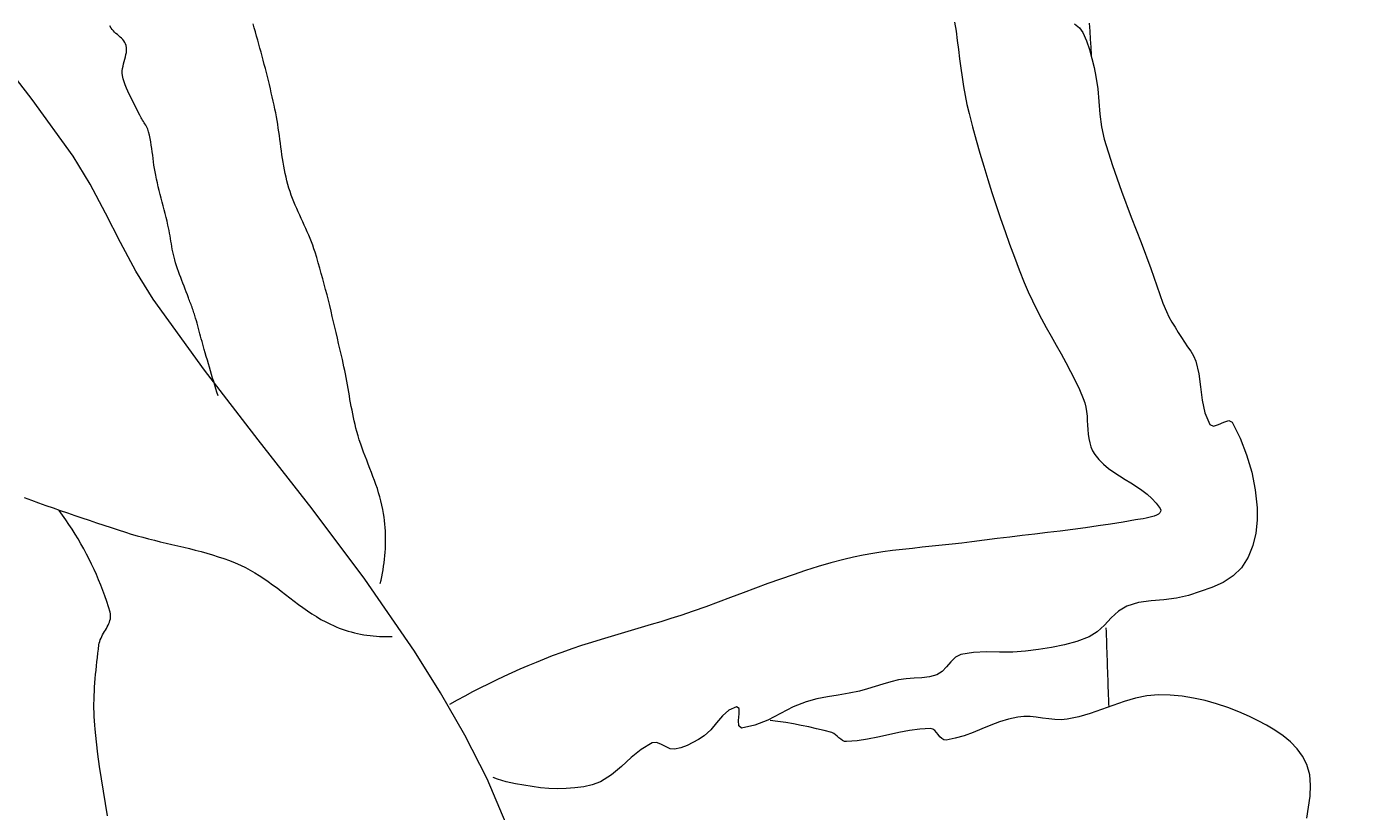
# Model space of a CAD drawing. Units: inches. Extents: x 1441 to 2460, y 1648 to 2683.
# Tile 7 of 35: x 1852 to 1880, y 1901 to 1917. Entities that reach past the tile are written whole.
import ezdxf

# ---------------------------------------------------------------- set-up
doc = ezdxf.new("R2010")
doc.units = ezdxf.units.IN
doc.layers.add('A-ANNO-DIMS', color=2, linetype='Continuous', lineweight=18)
doc.layers.add('A-FURN', color=8, linetype='Continuous', lineweight=15)
doc.styles.get("Standard").update_dxf_attribs({"font": 'arial.ttf'})
doc.dimstyles.get("Standard").update_dxf_attribs({"dimtxt": 0.18, "dimasz": 0.18, "dimexe": 0.18, "dimexo": 0.0625, "dimgap": 0.09, "dimtad": 0, "dimtih": 1, "dimtoh": 1, "dimdec": 4, "dimzin": 0, "dimdsep": 46, "dimtxsty": 'Standard', "dimcen": 0.09, "dimadec": 0, "dimazin": 0, "dimtfac": 1, "dimtdec": 4, "dimtofl": 0, "dimtmove": 0, "dimatfit": 3, "dimfxl": 1, "dimtolj": 1, "dimtzin": 0, "dimarcsym": 0})

# ---------------------------------------------------------------- blocks, each defined once
blk = doc.blocks.new('BED-DOUBLE-PLAN')
for p, q in [((30.489, 90.832), (30.333, 90.717)), ((30.661, 90.921), (30.489, 90.832)), ((30.874, 90.983), (30.661, 90.921)), ((31.094, 91.001), (30.874, 90.983)), ((31.32, 90.99), (31.094, 91.001)), ((31.549, 90.959), (31.32, 90.99)), ((31.78, 90.922), (31.549, 90.959)), ((30.192, 90.579), (30.063, 90.425)), ((30.333, 90.717), (30.192, 90.579)), ((29.947, 90.257), (29.842, 90.082)), ((30.063, 90.425), (29.947, 90.257)), ((29.842, 90.082), (29.747, 89.903)), ((23.852, 89.529), (24.202, 89.666)), ((24.202, 89.666), (24.563, 89.771)), ((24.563, 89.771), (24.931, 89.844)), ((24.931, 89.844), (25.302, 89.885)), ((25.302, 89.885), (25.565, 89.887)), ((25.565, 89.887), (25.831, 89.859)), ((25.831, 89.859), (26.09, 89.797)), ((26.09, 89.797), (26.334, 89.698)), ((26.334, 89.698), (26.554, 89.56)), ((29.66, 89.724), (29.561, 89.501)), ((29.747, 89.903), (29.66, 89.724)), ((23.52, 89.361), (23.852, 89.529)), ((26.554, 89.56), (26.727, 89.384)), ((26.727, 89.384), (26.861, 89.173)), ((29.561, 89.501), (29.471, 89.271)), ((23.486, 89.292), (23.52, 89.361)), ((23.516, 89.189), (23.486, 89.292)), ((23.569, 89.075), (23.516, 89.189)), ((26.861, 89.173), (26.965, 88.94)), ((29.471, 89.271), (29.393, 89.037)), ((23.32, 88.794), (23.566, 88.9)), ((23.566, 88.9), (23.6, 88.971)), ((23.6, 88.971), (23.569, 89.075)), ((26.965, 88.94), (27.052, 88.696)), ((29.393, 89.037), (29.327, 88.8)), ((22.037, 88.5), (22.136, 88.557)), ((22.136, 88.557), (22.241, 88.602)), ((22.241, 88.602), (22.507, 88.665)), ((22.507, 88.665), (22.781, 88.701)), ((22.781, 88.701), (23.055, 88.736)), ((23.055, 88.736), (23.32, 88.794)), ((27.052, 88.696), (27.132, 88.454)), ((29.274, 88.559), (29.236, 88.317)), ((29.327, 88.8), (29.274, 88.559)), ((21.643, 88.24), (21.75, 88.305)), ((21.75, 88.305), (21.847, 88.368)), ((21.847, 88.368), (21.942, 88.434)), ((21.942, 88.434), (22.037, 88.5)), ((27.132, 88.454), (27.192, 88.199)), ((29.236, 88.317), (29.214, 88.073)), ((21.031, 87.917), (21.207, 87.99)), ((21.207, 87.99), (21.32, 88.045)), ((21.32, 88.045), (21.429, 88.107)), ((21.429, 88.107), (21.536, 88.173)), ((21.536, 88.173), (21.643, 88.24)), ((27.192, 88.199), (27.223, 87.936)), ((29.214, 88.073), (29.208, 87.829)), ((20.309, 87.666), (20.489, 87.729)), ((20.489, 87.729), (20.67, 87.789)), ((20.67, 87.789), (20.851, 87.851)), ((20.851, 87.851), (21.031, 87.917)), ((25.019, 87.589), (25.108, 87.69)), ((25.108, 87.69), (25.206, 87.78)), ((25.206, 87.78), (25.316, 87.859)), ((25.316, 87.859), (25.351, 87.873)), ((25.351, 87.873), (25.382, 87.87)), ((25.382, 87.87), (25.41, 87.854)), ((25.41, 87.854), (25.435, 87.824)), ((25.435, 87.824), (25.457, 87.785)), ((25.457, 87.785), (25.476, 87.737)), ((25.476, 87.737), (25.493, 87.683)), ((27.223, 87.936), (27.246, 87.672)), ((29.208, 87.829), (29.229, 87.585)), ((19.236, 87.259), (19.771, 87.466)), ((19.771, 87.466), (20.309, 87.666)), ((24.859, 87.366), (24.936, 87.481)), ((24.936, 87.481), (25.019, 87.589)), ((25.493, 87.683), (25.508, 87.626)), ((25.508, 87.626), (25.521, 87.566)), ((25.521, 87.566), (25.532, 87.506)), ((25.532, 87.506), (25.542, 87.449)), ((25.542, 87.449), (25.551, 87.396)), ((27.246, 87.672), (27.284, 87.412)), ((27.284, 87.412), (27.359, 87.162)), ((29.229, 87.585), (29.278, 87.345)), ((18.7, 87.056), (19.236, 87.259)), ((24.638, 87.01), (24.712, 87.129)), ((24.712, 87.129), (24.785, 87.248)), ((24.785, 87.248), (24.859, 87.366)), ((25.551, 87.396), (25.559, 87.349)), ((25.559, 87.349), (25.604, 87.088)), ((27.359, 87.162), (27.462, 86.991)), ((29.278, 87.345), (29.347, 87.108)), ((17.613, 86.694), (18.16, 86.865)), ((18.16, 86.865), (18.7, 87.056)), ((24.481, 86.782), (24.562, 86.894)), ((24.562, 86.894), (24.638, 87.01)), ((25.604, 87.088), (25.646, 86.826)), ((27.462, 86.991), (27.601, 86.84)), ((29.347, 87.108), (29.428, 86.873)), ((29.428, 86.873), (29.514, 86.638)), ((16.564, 86.559), (16.828, 86.583)), ((16.828, 86.583), (17.093, 86.605)), ((17.093, 86.605), (17.356, 86.638)), ((17.356, 86.638), (17.613, 86.694)), ((24.194, 86.499), (24.299, 86.583)), ((24.299, 86.583), (24.394, 86.678)), ((24.394, 86.678), (24.481, 86.782)), ((25.646, 86.826), (25.684, 86.564)), ((27.601, 86.84), (27.752, 86.698)), ((27.752, 86.698), (27.893, 86.548)), ((27.813, 86.729), (27.896, 86.732)), ((27.896, 86.732), (27.979, 86.735)), ((27.979, 86.735), (28.061, 86.738)), ((28.061, 86.738), (28.144, 86.741)), ((28.144, 86.741), (28.226, 86.744)), ((28.226, 86.744), (28.309, 86.746)), ((28.309, 86.746), (28.391, 86.749)), ((28.391, 86.749), (28.474, 86.752)), ((28.474, 86.752), (28.556, 86.755)), ((28.556, 86.755), (28.639, 86.758)), ((28.639, 86.758), (28.722, 86.761)), ((28.722, 86.761), (28.804, 86.764)), ((28.804, 86.764), (28.887, 86.767)), ((28.887, 86.767), (28.969, 86.77)), ((28.969, 86.77), (29.052, 86.772)), ((29.052, 86.772), (29.134, 86.775)), ((29.134, 86.775), (29.217, 86.778)), ((29.217, 86.778), (29.3, 86.781)), ((29.3, 86.781), (29.382, 86.784)), ((29.382, 86.784), (29.465, 86.787)), ((29.514, 86.638), (29.596, 86.402)), ((15.193, 86.382), (15.36, 86.392)), ((15.36, 86.392), (15.527, 86.401)), ((15.385, 86.249), (15.56, 86.325)), ((15.527, 86.401), (15.694, 86.411)), ((15.56, 86.325), (15.741, 86.387)), ((15.694, 86.411), (15.86, 86.42)), ((15.741, 86.387), (15.927, 86.438)), ((15.927, 86.438), (16.114, 86.481)), ((16.114, 86.481), (16.302, 86.52)), ((16.302, 86.52), (16.564, 86.559)), ((23.026, 86.257), (23.113, 86.287)), ((23.113, 86.287), (23.203, 86.309)), ((23.203, 86.309), (23.295, 86.324)), ((23.295, 86.324), (23.389, 86.334)), ((23.389, 86.334), (23.483, 86.34)), ((23.483, 86.34), (23.578, 86.346)), ((23.578, 86.346), (23.673, 86.352)), ((23.673, 86.352), (23.767, 86.361)), ((23.767, 86.361), (23.858, 86.373)), ((23.858, 86.373), (23.948, 86.391)), ((23.948, 86.391), (24.034, 86.417)), ((24.034, 86.417), (24.116, 86.452)), ((24.116, 86.452), (24.194, 86.499)), ((25.684, 86.564), (25.721, 86.301)), ((25.721, 86.301), (25.756, 86.038)), ((27.893, 86.548), (28, 86.378)), ((28, 86.378), (28.096, 86.124)), ((29.596, 86.402), (29.666, 86.164)), ((15.205, 86.075), (15.287, 86.175)), ((15.287, 86.175), (15.385, 86.249)), ((22.459, 85.991), (22.646, 86.085)), ((22.646, 86.085), (22.835, 86.174)), ((22.835, 86.174), (23.026, 86.257)), ((25.756, 86.038), (25.789, 85.775)), ((28.096, 86.124), (28.167, 85.862)), ((29.666, 86.164), (29.717, 85.922)), ((21.908, 85.69), (22.091, 85.792)), ((22.091, 85.792), (22.274, 85.893)), ((22.274, 85.893), (22.459, 85.991)), ((25.789, 85.775), (25.821, 85.511)), ((28.167, 85.862), (28.22, 85.594)), ((29.717, 85.922), (29.728, 85.794)), ((29.728, 85.794), (29.724, 85.665)), ((21.358, 85.385), (21.542, 85.485)), ((21.542, 85.485), (21.725, 85.587)), ((21.725, 85.587), (21.908, 85.69)), ((25.821, 85.511), (25.853, 85.248)), ((28.22, 85.594), (28.261, 85.323)), ((29.71, 85.536), (29.692, 85.406)), ((29.724, 85.665), (29.71, 85.536)), ((20.796, 85.106), (20.986, 85.194)), ((20.986, 85.194), (21.173, 85.287)), ((21.173, 85.287), (21.358, 85.385)), ((25.853, 85.248), (25.884, 84.984)), ((28.261, 85.323), (28.298, 85.053)), ((29.674, 85.276), (29.661, 85.147)), ((29.692, 85.406), (29.674, 85.276)), ((20.072, 84.818), (20.338, 84.92)), ((20.338, 84.92), (20.604, 85.025)), ((20.604, 85.025), (20.796, 85.106)), ((25.884, 84.984), (25.915, 84.72)), ((28.298, 85.053), (28.318, 84.783)), ((29.661, 85.147), (29.658, 85.018)), ((29.658, 85.018), (29.671, 84.89)), ((29.671, 84.89), (29.714, 84.699)), ((19.265, 84.529), (19.535, 84.623)), ((19.535, 84.623), (19.804, 84.719)), ((19.804, 84.719), (20.072, 84.818)), ((25.915, 84.72), (25.948, 84.457)), ((28.318, 84.783), (28.316, 84.51)), ((29.714, 84.699), (29.774, 84.511)), ((18.451, 84.264), (18.723, 84.35)), ((18.723, 84.35), (18.995, 84.438)), ((18.995, 84.438), (19.265, 84.529)), ((25.948, 84.457), (25.981, 84.194)), ((28.316, 84.51), (28.311, 84.238)), ((29.774, 84.511), (29.844, 84.326)), ((29.844, 84.326), (29.919, 84.142)), ((17.629, 84.022), (17.903, 84.1)), ((17.903, 84.1), (18.177, 84.181)), ((18.177, 84.181), (18.451, 84.264)), ((25.981, 84.194), (26.015, 83.931)), ((28.311, 84.238), (28.322, 83.968)), ((29.919, 84.142), (29.993, 83.958)), ((16.51, 83.755), (16.701, 83.789)), ((16.701, 83.789), (16.89, 83.828)), ((16.89, 83.828), (17.078, 83.873)), ((17.078, 83.873), (17.353, 83.946)), ((17.353, 83.946), (17.629, 84.022)), ((26.015, 83.931), (26.042, 83.725)), ((28.322, 83.968), (28.367, 83.704)), ((29.993, 83.958), (30.06, 83.772)), ((30.06, 83.772), (30.115, 83.584)), ((15.168, 83.572), (15.359, 83.6)), ((15.359, 83.6), (15.551, 83.626)), ((15.551, 83.626), (15.743, 83.651)), ((15.743, 83.651), (15.935, 83.675)), ((15.935, 83.675), (16.128, 83.699)), ((16.128, 83.699), (16.319, 83.726)), ((16.319, 83.726), (16.51, 83.755)), ((26.042, 83.725), (26.065, 83.518)), ((26.065, 83.518), (26.087, 83.311)), ((28.367, 83.704), (28.424, 83.589)), ((28.424, 83.589), (28.516, 83.493)), ((28.516, 83.493), (28.62, 83.403)), ((30.115, 83.584), (30.152, 83.392)), ((26.087, 83.311), (26.108, 83.104)), ((28.62, 83.403), (28.718, 83.309)), ((28.718, 83.309), (28.788, 83.198)), ((30.037, 83.229), (29.991, 83.193)), ((30.083, 83.265), (30.037, 83.229)), ((30.121, 83.303), (30.083, 83.265)), ((30.146, 83.345), (30.121, 83.303)), ((30.152, 83.392), (30.146, 83.345)), ((26.108, 83.104), (26.129, 82.897)), ((28.788, 83.198), (28.833, 83.045)), ((28.833, 83.045), (28.854, 82.886)), ((29.921, 83.113), (29.911, 83.066)), ((29.911, 83.066), (29.924, 82.845)), ((29.95, 83.155), (29.921, 83.113)), ((29.991, 83.193), (29.95, 83.155)), ((26.129, 82.897), (26.151, 82.689)), ((26.151, 82.689), (26.173, 82.483)), ((28.854, 82.886), (28.863, 82.724)), ((28.863, 82.724), (28.873, 82.561)), ((29.924, 82.845), (29.954, 82.626)), ((26.173, 82.483), (26.198, 82.276)), ((28.873, 82.561), (28.896, 82.401)), ((28.896, 82.401), (28.937, 82.237)), ((29.954, 82.626), (29.995, 82.407)), ((29.995, 82.407), (30.042, 82.189)), ((26.198, 82.276), (26.226, 82.07)), ((28.937, 82.237), (28.985, 82.075)), ((30.042, 82.189), (30.09, 81.971)), ((26.226, 82.07), (26.258, 81.865)), ((26.258, 81.865), (26.294, 81.661)), ((28.985, 82.075), (29.036, 81.914)), ((29.036, 81.914), (29.086, 81.753)), ((30.09, 81.971), (30.133, 81.753)), ((26.294, 81.661), (26.335, 81.458)), ((29.086, 81.753), (29.129, 81.589)), ((29.129, 81.589), (29.175, 81.367)), ((30.133, 81.753), (30.166, 81.534)), ((30.166, 81.534), (30.185, 81.313)), ((26.335, 81.458), (26.383, 81.256)), ((26.383, 81.256), (26.454, 80.989)), ((29.175, 81.367), (29.213, 81.142)), ((30.179, 81.27), (30.162, 81.231)), ((30.185, 81.313), (30.179, 81.27)), ((26.454, 80.989), (26.531, 80.724)), ((29.213, 81.142), (29.25, 80.917)), ((29.996, 81.006), (29.954, 80.848)), ((30.014, 81.048), (29.996, 81.006)), ((30.04, 81.086), (30.014, 81.048)), ((30.071, 81.123), (30.04, 81.086)), ((30.104, 81.158), (30.071, 81.123)), ((30.136, 81.194), (30.104, 81.158)), ((30.162, 81.231), (30.136, 81.194)), ((26.531, 80.724), (26.614, 80.46)), ((29.25, 80.917), (29.294, 80.695)), ((29.294, 80.695), (29.352, 80.475)), ((29.915, 80.689), (29.879, 80.529)), ((29.954, 80.848), (29.915, 80.689)), ((26.614, 80.46), (26.702, 80.198)), ((29.352, 80.475), (29.461, 80.202)), ((29.879, 80.529), (29.846, 80.368)), ((26.702, 80.198), (26.793, 79.936)), ((29.461, 80.202), (29.597, 79.937)), ((29.815, 80.207), (29.788, 80.045)), ((29.846, 80.368), (29.815, 80.207)), ((26.793, 79.936), (26.887, 79.676)), ((29.597, 79.937), (29.734, 79.673)), ((29.764, 79.883), (29.743, 79.721)), ((29.788, 80.045), (29.764, 79.883)), ((26.887, 79.676), (26.983, 79.416)), ((29.734, 79.673), (29.843, 79.403)), ((26.983, 79.416), (27.08, 79.157)), ((29.843, 79.403), (29.9, 79.12)), ((27.08, 79.157), (27.177, 78.897)), ((29.494, 79.073), (29.458, 79.021)), ((29.458, 79.021), (29.528, 78.86)), ((29.604, 79.076), (29.494, 79.073)), ((29.741, 79.063), (29.604, 79.076)), ((29.856, 79.066), (29.741, 79.063)), ((29.9, 79.12), (29.856, 79.066)), ((27.177, 78.897), (27.274, 78.638)), ((29.528, 78.86), (29.648, 78.726)), ((29.648, 78.726), (29.793, 78.603)), ((27.274, 78.638), (27.368, 78.377)), ((29.793, 78.603), (29.939, 78.48)), ((29.939, 78.48), (30.061, 78.342)), ((27.368, 78.377), (27.461, 78.116)), ((30.061, 78.342), (30.137, 78.228)), ((30.137, 78.228), (30.206, 78.109)), ((27.461, 78.116), (27.55, 77.854)), ((30.206, 78.109), (30.267, 77.986)), ((30.267, 77.986), (30.314, 77.859)), ((27.55, 77.854), (27.616, 77.649)), ((27.616, 77.649), (27.681, 77.442)), ((30.332, 77.631), (30.288, 77.537)), ((30.314, 77.859), (30.343, 77.727)), ((30.343, 77.727), (30.332, 77.631)), ((27.681, 77.442), (27.743, 77.235)), ((30.237, 77.443), (30.203, 77.351)), ((30.203, 77.351), (30.212, 77.262)), ((30.288, 77.537), (30.237, 77.443)), ((27.743, 77.235), (27.805, 77.028)), ((30.212, 77.262), (30.347, 77.03)), ((27.805, 77.028), (27.866, 76.82)), ((27.866, 76.82), (27.927, 76.612)), ((30.347, 77.03), (30.518, 76.819)), ((30.518, 76.819), (30.704, 76.617)), ((27.927, 76.612), (27.988, 76.405)), ((30.704, 76.617), (30.879, 76.408)), ((27.988, 76.405), (28.051, 76.197)), ((30.879, 76.408), (31.02, 76.18)), ((28.051, 76.197), (28.114, 75.991)), ((28.114, 75.991), (28.18, 75.785)), ((31.02, 76.18), (31.086, 76.009)), ((31.086, 76.009), (31.127, 75.831)), ((28.18, 75.785), (28.249, 75.58)), ((31.127, 75.831), (31.15, 75.647)), ((31.15, 75.647), (31.161, 75.461)), ((28.249, 75.58), (28.321, 75.376)), ((28.321, 75.376), (28.397, 75.174)), ((31.161, 75.461), (31.167, 75.277)), ((28.397, 75.174), (28.463, 75.004)), ((31.164, 75.101), (31.148, 74.926)), ((31.167, 75.277), (31.164, 75.101)), ((28.463, 75.004), (28.532, 74.835)), ((28.532, 74.835), (28.602, 74.666)), ((31.148, 74.926), (31.124, 74.751)), ((28.602, 74.666), (28.675, 74.499)), ((31.094, 74.577), (31.064, 74.403)), ((31.124, 74.751), (31.094, 74.577)), ((28.675, 74.499), (28.749, 74.332)), ((28.749, 74.332), (28.825, 74.166)), ((31.045, 74.308), (31.023, 74.214)), ((31.064, 74.403), (31.045, 74.308)), ((28.825, 74.166), (28.903, 74.001)), ((28.903, 74.001), (28.983, 73.837)), ((30.966, 74.029), (30.933, 73.938)), ((31.901, 74.215), (30.964, 73.813)), ((30.996, 74.121), (30.966, 74.029)), ((31.023, 74.214), (30.996, 74.121)), ((28.983, 73.837), (29.064, 73.674)), ((30.964, 73.813), (30.052, 73.35)), ((29.064, 73.674), (29.148, 73.511)), ((29.148, 73.511), (29.233, 73.35)), ((30.052, 73.35), (29.164, 72.842)), ((29.233, 73.35), (29.32, 73.189)), ((29.32, 73.189), (29.409, 73.03)), ((29.164, 72.842), (28.298, 72.301)), ((28.298, 72.301), (26.791, 71.264)), ((27.992, 71.766), (27.99, 71.832)), ((27.993, 71.7), (27.992, 71.766)), ((24.735, 71.463), (24.65, 71.431)), ((24.819, 71.493), (24.735, 71.463)), ((24.904, 71.523), (24.819, 71.493)), ((24.99, 71.55), (24.904, 71.523)), ((25.076, 71.576), (24.99, 71.55)), ((25.162, 71.599), (25.076, 71.576)), ((25.25, 71.62), (25.162, 71.599)), ((25.337, 71.638), (25.25, 71.62)), ((25.426, 71.654), (25.337, 71.638)), ((25.498, 71.664), (25.426, 71.654)), ((25.571, 71.673), (25.498, 71.664)), ((25.644, 71.68), (25.571, 71.673)), ((25.717, 71.686), (25.644, 71.68)), ((25.79, 71.691), (25.717, 71.686)), ((25.864, 71.694), (25.79, 71.691)), ((25.938, 71.695), (25.864, 71.694)), ((26.011, 71.695), (25.938, 71.695)), ((26.085, 71.694), (26.011, 71.695)), ((26.159, 71.691), (26.085, 71.694)), ((26.233, 71.687), (26.159, 71.691)), ((26.306, 71.681), (26.233, 71.687)), ((26.379, 71.674), (26.306, 71.681)), ((26.453, 71.665), (26.379, 71.674)), ((26.525, 71.655), (26.453, 71.665)), ((26.598, 71.643), (26.525, 71.655)), ((26.67, 71.63), (26.598, 71.643)), ((26.742, 71.616), (26.67, 71.63)), ((26.814, 71.6), (26.742, 71.616)), ((26.885, 71.583), (26.814, 71.6)), ((27.98, 71.436), (27.985, 71.502)), ((27.985, 71.502), (27.99, 71.568)), ((27.99, 71.568), (27.992, 71.634)), ((27.992, 71.634), (27.993, 71.7)), ((23.974, 71.176), (23.888, 71.147)), ((24.059, 71.205), (23.974, 71.176)), ((24.144, 71.236), (24.059, 71.205)), ((24.228, 71.268), (24.144, 71.236)), ((24.313, 71.301), (24.228, 71.268)), ((24.397, 71.334), (24.313, 71.301)), ((24.481, 71.366), (24.397, 71.334)), ((24.566, 71.399), (24.481, 71.366)), ((24.65, 71.431), (24.566, 71.399)), ((26.791, 71.264), (25.327, 70.164)), ((27.927, 71.108), (27.941, 71.173)), ((27.941, 71.173), (27.953, 71.239)), ((27.953, 71.239), (27.964, 71.304)), ((27.964, 71.304), (27.972, 71.37)), ((27.972, 71.37), (27.98, 71.436)), ((22.663, 70.885), (22.588, 70.871)), ((22.739, 70.899), (22.663, 70.885)), ((22.814, 70.912), (22.739, 70.899)), ((22.89, 70.926), (22.814, 70.912)), ((22.965, 70.939), (22.89, 70.926)), ((23.041, 70.952), (22.965, 70.939)), ((23.116, 70.966), (23.041, 70.952)), ((23.192, 70.98), (23.116, 70.966)), ((23.267, 70.995), (23.192, 70.98)), ((23.342, 71.01), (23.267, 70.995)), ((23.417, 71.025), (23.342, 71.01)), ((23.492, 71.042), (23.417, 71.025)), ((23.567, 71.059), (23.492, 71.042)), ((23.641, 71.077), (23.567, 71.059)), ((23.715, 71.097), (23.641, 71.077)), ((23.802, 71.121), (23.715, 71.097)), ((23.888, 71.147), (23.802, 71.121)), ((27.858, 70.852), (27.877, 70.915)), ((27.877, 70.915), (27.895, 70.979)), ((27.895, 70.979), (27.912, 71.044)), ((27.912, 71.044), (27.927, 71.108)), ((21.423, 70.61), (21.31, 70.583)), ((21.536, 70.636), (21.423, 70.61)), ((21.648, 70.663), (21.536, 70.636)), ((21.761, 70.689), (21.648, 70.663)), ((21.874, 70.715), (21.761, 70.689)), ((21.987, 70.741), (21.874, 70.715)), ((22.1, 70.767), (21.987, 70.741)), ((22.212, 70.793), (22.1, 70.767)), ((22.287, 70.81), (22.212, 70.793)), ((22.362, 70.827), (22.287, 70.81)), ((22.437, 70.842), (22.362, 70.827)), ((22.512, 70.857), (22.437, 70.842)), ((22.588, 70.871), (22.512, 70.857)), ((27.736, 70.546), (27.764, 70.606)), ((27.764, 70.606), (27.789, 70.666)), ((27.789, 70.666), (27.814, 70.727)), ((27.814, 70.727), (27.836, 70.79)), ((27.836, 70.79), (27.858, 70.852)), ((20.302, 70.323), (20.191, 70.29)), ((20.413, 70.354), (20.302, 70.323)), ((20.525, 70.385), (20.413, 70.354)), ((20.636, 70.415), (20.525, 70.385)), ((20.748, 70.444), (20.636, 70.415)), ((20.861, 70.473), (20.748, 70.444)), ((20.973, 70.501), (20.861, 70.473)), ((21.085, 70.529), (20.973, 70.501)), ((21.198, 70.556), (21.085, 70.529)), ((21.31, 70.583), (21.198, 70.556)), ((27.576, 70.251), (27.633, 70.347)), ((27.633, 70.347), (27.687, 70.445)), ((27.687, 70.445), (27.736, 70.546)), ((19.544, 70.06), (19.475, 70.029)), ((19.614, 70.091), (19.544, 70.06)), ((19.684, 70.12), (19.614, 70.091)), ((19.754, 70.148), (19.684, 70.12)), ((19.825, 70.175), (19.754, 70.148)), ((19.897, 70.2), (19.825, 70.175)), ((19.969, 70.223), (19.897, 70.2)), ((20.08, 70.257), (19.969, 70.223)), ((20.191, 70.29), (20.08, 70.257)), ((25.327, 70.164), (23.883, 69.037)), ((27.387, 69.97), (27.452, 70.062)), ((27.452, 70.062), (27.515, 70.156)), ((27.515, 70.156), (27.576, 70.251)), ((18.919, 69.781), (18.848, 69.753)), ((18.989, 69.81), (18.919, 69.781)), ((19.059, 69.841), (18.989, 69.81)), ((19.128, 69.871), (19.059, 69.841)), ((19.197, 69.903), (19.128, 69.871)), ((19.267, 69.935), (19.197, 69.903)), ((19.336, 69.966), (19.267, 69.935)), ((19.405, 69.998), (19.336, 69.966)), ((19.475, 70.029), (19.405, 69.998)), ((27.184, 69.699), (27.253, 69.789)), ((27.253, 69.789), (27.321, 69.879)), ((27.321, 69.879), (27.387, 69.97)), ((17.538, 69.478), (17.459, 69.467)), ((17.618, 69.488), (17.538, 69.478)), ((17.697, 69.499), (17.618, 69.488)), ((17.777, 69.509), (17.697, 69.499)), ((17.856, 69.52), (17.777, 69.509)), ((17.935, 69.531), (17.856, 69.52)), ((18.014, 69.543), (17.935, 69.531)), ((18.093, 69.555), (18.014, 69.543)), ((18.172, 69.569), (18.093, 69.555)), ((18.25, 69.583), (18.172, 69.569)), ((18.329, 69.599), (18.25, 69.583)), ((18.407, 69.617), (18.329, 69.599)), ((18.484, 69.635), (18.407, 69.617)), ((18.561, 69.656), (18.484, 69.635)), ((18.634, 69.678), (18.561, 69.656)), ((18.706, 69.701), (18.634, 69.678)), ((18.777, 69.726), (18.706, 69.701)), ((18.848, 69.753), (18.777, 69.726)), ((26.978, 69.429), (27.046, 69.519)), ((27.046, 69.519), (27.115, 69.609)), ((27.115, 69.609), (27.184, 69.699)), ((16.219, 69.207), (16.134, 69.186)), ((16.304, 69.228), (16.219, 69.207)), ((16.389, 69.249), (16.304, 69.228)), ((16.474, 69.27), (16.389, 69.249)), ((16.559, 69.29), (16.474, 69.27)), ((16.644, 69.31), (16.559, 69.29)), ((16.73, 69.33), (16.644, 69.31)), ((16.815, 69.349), (16.73, 69.33)), ((16.901, 69.368), (16.815, 69.349)), ((16.986, 69.387), (16.901, 69.368)), ((17.064, 69.403), (16.986, 69.387)), ((17.143, 69.417), (17.064, 69.403)), ((17.222, 69.431), (17.143, 69.417)), ((17.301, 69.444), (17.222, 69.431)), ((17.38, 69.456), (17.301, 69.444)), ((17.459, 69.467), (17.38, 69.456)), ((26.78, 69.154), (26.844, 69.246)), ((26.844, 69.246), (26.91, 69.338)), ((26.91, 69.338), (26.978, 69.429)), ((15.29, 68.954), (15.204, 68.929)), ((15.375, 68.979), (15.29, 68.954)), ((15.459, 69.003), (15.375, 68.979)), ((15.543, 69.026), (15.459, 69.003)), ((15.627, 69.05), (15.543, 69.026)), ((15.711, 69.073), (15.627, 69.05)), ((15.796, 69.096), (15.711, 69.073)), ((15.88, 69.119), (15.796, 69.096)), ((15.965, 69.142), (15.88, 69.119)), ((16.05, 69.164), (15.965, 69.142)), ((16.134, 69.186), (16.05, 69.164)), ((23.883, 69.037), (22.432, 67.918)), ((26.603, 68.868), (26.659, 68.965)), ((26.659, 68.965), (26.718, 69.06)), ((26.718, 69.06), (26.78, 69.154)), ((26.453, 68.553), (26.503, 68.668)), ((26.503, 68.668), (26.551, 68.769)), ((26.551, 68.769), (26.603, 68.868)), ((26.365, 68.321), (26.407, 68.437)), ((26.407, 68.437), (26.453, 68.553)), ((22.596, 68.086), (22.521, 68.063)), ((22.671, 68.108), (22.596, 68.086)), ((22.745, 68.131), (22.671, 68.108)), ((22.82, 68.154), (22.745, 68.131)), ((22.894, 68.176), (22.82, 68.154)), ((22.969, 68.199), (22.894, 68.176)), ((26.252, 67.965), (26.287, 68.084)), ((26.287, 68.084), (26.325, 68.203)), ((26.325, 68.203), (26.365, 68.321)), ((22.432, 67.918), (20.949, 66.844)), ((21.617, 67.806), (21.563, 67.791)), ((21.672, 67.82), (21.617, 67.806)), ((21.726, 67.835), (21.672, 67.82)), ((21.781, 67.849), (21.726, 67.835)), ((21.835, 67.864), (21.781, 67.849)), ((21.89, 67.879), (21.835, 67.864)), ((21.944, 67.894), (21.89, 67.879)), ((21.998, 67.909), (21.944, 67.894)), ((22.073, 67.931), (21.998, 67.909)), ((22.148, 67.953), (22.073, 67.931)), ((22.223, 67.975), (22.148, 67.953)), ((22.297, 67.997), (22.223, 67.975)), ((22.372, 68.019), (22.297, 67.997)), ((22.447, 68.041), (22.372, 68.019)), ((22.521, 68.063), (22.447, 68.041)), ((26.187, 67.724), (26.219, 67.844)), ((26.219, 67.844), (26.252, 67.965)), ((20.8, 67.536), (20.74, 67.513)), ((20.861, 67.559), (20.8, 67.536)), ((20.922, 67.581), (20.861, 67.559)), ((20.95, 67.591), (20.922, 67.581)), ((20.979, 67.602), (20.95, 67.591)), ((21.007, 67.612), (20.979, 67.602)), ((21.036, 67.623), (21.007, 67.612)), ((21.064, 67.634), (21.036, 67.623)), ((21.092, 67.645), (21.064, 67.634)), ((21.12, 67.655), (21.092, 67.645)), ((21.149, 67.666), (21.12, 67.655)), ((21.177, 67.676), (21.149, 67.666)), ((21.206, 67.686), (21.177, 67.676)), ((21.234, 67.696), (21.206, 67.686)), ((21.263, 67.705), (21.234, 67.696)), ((21.292, 67.714), (21.263, 67.705)), ((21.346, 67.73), (21.292, 67.714)), ((21.4, 67.746), (21.346, 67.73)), ((21.454, 67.761), (21.4, 67.746)), ((21.509, 67.776), (21.454, 67.761)), ((21.563, 67.791), (21.509, 67.776)), ((26.127, 67.481), (26.156, 67.602)), ((26.156, 67.602), (26.187, 67.724)), ((19.908, 67.244), (19.852, 67.234)), ((19.964, 67.255), (19.908, 67.244)), ((20.019, 67.267), (19.964, 67.255)), ((20.074, 67.28), (20.019, 67.267)), ((20.129, 67.295), (20.074, 67.28)), ((20.191, 67.313), (20.129, 67.295)), ((20.253, 67.333), (20.191, 67.313)), ((20.315, 67.353), (20.253, 67.333)), ((20.376, 67.375), (20.315, 67.353)), ((20.437, 67.397), (20.376, 67.375)), ((20.498, 67.419), (20.437, 67.397)), ((20.558, 67.442), (20.498, 67.419)), ((20.619, 67.466), (20.558, 67.442)), ((20.679, 67.489), (20.619, 67.466)), ((20.74, 67.513), (20.679, 67.489)), ((26.041, 67.115), (26.069, 67.237)), ((26.069, 67.237), (26.098, 67.359)), ((26.098, 67.359), (26.127, 67.481)), ((18.683, 66.971), (18.603, 66.951)), ((18.764, 66.991), (18.683, 66.971)), ((18.843, 67.012), (18.764, 66.991)), ((18.923, 67.033), (18.843, 67.012)), ((19.003, 67.054), (18.923, 67.033)), ((19.083, 67.074), (19.003, 67.054)), ((19.163, 67.095), (19.083, 67.074)), ((19.243, 67.115), (19.163, 67.095)), ((19.324, 67.134), (19.243, 67.115)), ((19.404, 67.153), (19.324, 67.134)), ((19.46, 67.165), (19.404, 67.153)), ((19.515, 67.176), (19.46, 67.165)), ((19.571, 67.186), (19.515, 67.176)), ((19.628, 67.196), (19.571, 67.186)), ((19.684, 67.205), (19.628, 67.196)), ((19.74, 67.214), (19.684, 67.205)), ((19.796, 67.224), (19.74, 67.214)), ((19.852, 67.234), (19.796, 67.224)), ((25.982, 66.871), (26.012, 66.993)), ((26.012, 66.993), (26.041, 67.115)), ((17.32, 66.689), (17.294, 66.673)), ((17.347, 66.704), (17.32, 66.689)), ((17.374, 66.718), (17.347, 66.704)), ((17.402, 66.73), (17.374, 66.718)), ((17.43, 66.741), (17.402, 66.73)), ((17.459, 66.75), (17.43, 66.741)), ((17.527, 66.767), (17.459, 66.75)), ((17.596, 66.782), (17.527, 66.767)), ((17.665, 66.794), (17.596, 66.782)), ((17.734, 66.806), (17.665, 66.794)), ((17.804, 66.816), (17.734, 66.806)), ((17.874, 66.825), (17.804, 66.816)), ((17.944, 66.834), (17.874, 66.825)), ((18.014, 66.843), (17.944, 66.834)), ((18.084, 66.851), (18.014, 66.843)), ((18.154, 66.861), (18.084, 66.851)), ((18.223, 66.871), (18.154, 66.861)), ((18.293, 66.883), (18.223, 66.871)), ((18.362, 66.897), (18.293, 66.883)), ((18.443, 66.914), (18.362, 66.897)), ((18.523, 66.932), (18.443, 66.914)), ((18.603, 66.951), (18.523, 66.932)), ((20.949, 66.844), (20.369, 66.483)), ((25.92, 66.629), (25.952, 66.75)), ((25.952, 66.75), (25.982, 66.871)), ((16.797, 66.407), (16.734, 66.375)), ((16.859, 66.439), (16.797, 66.407)), ((16.921, 66.471), (16.859, 66.439)), ((16.983, 66.503), (16.921, 66.471)), ((17.045, 66.534), (16.983, 66.503)), ((17.108, 66.564), (17.045, 66.534)), ((17.136, 66.577), (17.108, 66.564)), ((17.163, 66.592), (17.136, 66.577)), ((17.189, 66.608), (17.163, 66.592)), ((17.215, 66.624), (17.189, 66.608)), ((17.241, 66.64), (17.215, 66.624)), ((17.268, 66.657), (17.241, 66.64)), ((17.294, 66.673), (17.268, 66.657)), ((20.369, 66.483), (19.765, 66.161)), ((25.852, 66.388), (25.887, 66.508)), ((25.887, 66.508), (25.92, 66.629)), ((15.455, 66.127), (15.43, 66.097)), ((15.481, 66.156), (15.455, 66.127)), ((15.506, 66.183), (15.481, 66.156)), ((15.533, 66.209), (15.506, 66.183)), ((15.561, 66.233), (15.533, 66.209)), ((15.591, 66.253), (15.561, 66.233)), ((15.623, 66.268), (15.591, 66.253)), ((15.658, 66.28), (15.623, 66.268)), ((15.705, 66.287), (15.658, 66.28)), ((15.752, 66.289), (15.705, 66.287)), ((15.8, 66.285), (15.752, 66.289)), ((15.848, 66.277), (15.8, 66.285)), ((15.896, 66.266), (15.848, 66.277)), ((15.945, 66.253), (15.896, 66.266)), ((15.993, 66.239), (15.945, 66.253)), ((16.042, 66.226), (15.993, 66.239)), ((16.09, 66.215), (16.042, 66.226)), ((16.138, 66.206), (16.09, 66.215)), ((16.186, 66.2), (16.138, 66.206)), ((16.234, 66.2), (16.186, 66.2)), ((16.282, 66.206), (16.234, 66.2)), ((16.349, 66.221), (16.282, 66.206)), ((16.415, 66.24), (16.349, 66.221)), ((16.48, 66.263), (16.415, 66.24)), ((16.545, 66.288), (16.48, 66.263)), ((16.609, 66.315), (16.545, 66.288)), ((16.672, 66.344), (16.609, 66.315)), ((16.734, 66.375), (16.672, 66.344)), ((19.765, 66.161), (19.153, 65.853)), ((25.716, 65.966), (25.765, 66.117)), ((25.765, 66.117), (25.815, 66.269)), ((25.815, 66.269), (25.852, 66.388)), ((15.292, 65.969), (15.247, 65.942)), ((15.323, 65.99), (15.292, 65.969)), ((15.351, 66.014), (15.323, 65.99)), ((15.379, 66.04), (15.351, 66.014)), ((15.405, 66.068), (15.379, 66.04)), ((15.43, 66.097), (15.405, 66.068)), ((19.153, 65.853), (18.549, 65.531)), ((25.666, 65.814), (25.716, 65.966)), ((27.145, 65.835), (27.033, 65.794)), ((27.257, 65.874), (27.145, 65.835)), ((27.37, 65.911), (27.257, 65.874)), ((27.484, 65.946), (27.37, 65.911)), ((27.519, 65.953), (27.484, 65.946)), ((27.553, 65.957), (27.519, 65.953)), ((27.587, 65.955), (27.553, 65.957)), ((27.62, 65.951), (27.587, 65.955)), ((27.654, 65.942), (27.62, 65.951)), ((27.688, 65.931), (27.654, 65.942)), ((27.721, 65.918), (27.688, 65.931)), ((27.755, 65.902), (27.721, 65.918)), ((27.788, 65.885), (27.755, 65.902)), ((27.822, 65.867), (27.788, 65.885)), ((27.855, 65.847), (27.822, 65.867)), ((27.889, 65.828), (27.855, 65.847)), ((31.475, 65.847), (31.218, 65.805)), ((31.732, 65.891), (31.475, 65.847)), ((25.566, 65.51), (25.616, 65.662)), ((25.616, 65.662), (25.666, 65.814)), ((26.483, 65.559), (26.375, 65.506)), ((26.591, 65.61), (26.483, 65.559)), ((26.7, 65.659), (26.591, 65.61)), ((26.81, 65.706), (26.7, 65.659)), ((26.921, 65.751), (26.81, 65.706)), ((27.033, 65.794), (26.921, 65.751)), ((27.923, 65.809), (27.889, 65.828)), ((27.957, 65.79), (27.923, 65.809)), ((27.991, 65.772), (27.957, 65.79)), ((28.025, 65.756), (27.991, 65.772)), ((28.06, 65.741), (28.025, 65.756)), ((28.094, 65.729), (28.06, 65.741)), ((28.13, 65.72), (28.094, 65.729)), ((28.165, 65.713), (28.13, 65.72)), ((28.253, 65.702), (28.165, 65.713)), ((28.34, 65.691), (28.253, 65.702)), ((28.428, 65.681), (28.34, 65.691)), ((28.516, 65.67), (28.428, 65.681)), ((28.604, 65.661), (28.516, 65.67)), ((28.692, 65.652), (28.604, 65.661)), ((28.78, 65.643), (28.692, 65.652)), ((28.869, 65.635), (28.78, 65.643)), ((28.957, 65.628), (28.869, 65.635)), ((29.045, 65.622), (28.957, 65.628)), ((29.133, 65.617), (29.045, 65.622)), ((29.222, 65.613), (29.133, 65.617)), ((29.31, 65.611), (29.222, 65.613)), ((29.398, 65.609), (29.31, 65.611)), ((29.487, 65.609), (29.398, 65.609)), ((29.575, 65.61), (29.487, 65.609)), ((29.663, 65.613), (29.575, 65.61)), ((29.751, 65.618), (29.663, 65.613)), ((29.839, 65.624), (29.751, 65.618)), ((29.927, 65.632), (29.839, 65.624)), ((30.186, 65.66), (29.927, 65.632)), ((30.444, 65.692), (30.186, 65.66)), ((30.702, 65.727), (30.444, 65.692)), ((30.96, 65.765), (30.702, 65.727)), ((31.218, 65.805), (30.96, 65.765)), ((18.549, 65.531), (17.968, 65.172)), ((25.464, 65.207), (25.515, 65.359)), ((25.515, 65.359), (25.566, 65.51)), ((25.955, 65.277), (25.853, 65.215)), ((26.059, 65.337), (25.955, 65.277)), ((26.163, 65.395), (26.059, 65.337)), ((26.269, 65.452), (26.163, 65.395)), ((26.375, 65.506), (26.269, 65.452)), ((17.968, 65.172), (16.787, 64.32)), ((25.361, 64.905), (25.413, 65.056)), ((25.413, 65.056), (25.464, 65.207)), ((25.553, 65.02), (25.456, 64.951)), ((25.652, 65.087), (25.553, 65.02)), ((25.752, 65.152), (25.652, 65.087)), ((25.853, 65.215), (25.752, 65.152)), ((25.256, 64.603), (25.308, 64.754)), ((25.308, 64.754), (25.361, 64.905)), ((25.456, 64.951), (25.36, 64.881)), ((25.148, 64.303), (25.202, 64.453)), ((25.202, 64.453), (25.256, 64.603)), ((16.787, 64.32), (15.632, 63.429)), ((25.093, 64.152), (25.148, 64.303))]:
    blk.add_line(p, q)
blk = doc.blocks.new('*D67')
at = {"layer": 'A-ANNO-DIMS', "color": 0, "lineweight": -2, "transparency": 16777216}
for p, q in [((1889.448, 2298.695), (1916.216, 2298.695)), ((1916.036, 2298.515), (1916.036, 2055.938)), ((1916.036, 1812.997), (1916.036, 2055.574)), ((1758.224, 1812.817), (1916.216, 1812.817))]:
    blk.add_line(p, q, dxfattribs=at)
at = {"layer": 'A-ANNO-DIMS', "color": 0, "transparency": 16777216}
for points in [[(1916.006, 2298.515), (1916.066, 2298.515), (1916.036, 2298.695)], [(1916.006, 1812.997), (1916.066, 1812.997), (1916.036, 1812.817)]]:
    blk.add_solid(points, dxfattribs=at)
at = {"layer": 'Defpoints', "color": 0, "transparency": 16777216}
for p in [(1889.386, 2298.695), (1916.036, 2298.695), (1758.161, 1812.817)]:
    blk.add_point(p, dxfattribs=at)
at = {"layer": 'A-ANNO-DIMS', "color": 0, "transparency": 16777216, "insert": (1916.036, 2055.756), "char_height": 0.18, "attachment_point": 5}
blk.add_mtext('\\A1;485.9', dxfattribs=at)

msp = doc.modelspace()

# ---------------------------------------------------------------- block references
at = {"layer": 'A-FURN', "rotation": 270}
msp.add_blockref('BED-DOUBLE-PLAN', (1787.6309, 1932.2861), dxfattribs=at)

# ---------------------------------------------------------------- dimensions: what is measured, and where the dimension line sits
at = {"layer": 'A-ANNO-DIMS'}
dim = msp.add_linear_dim(base=(1916.0359, 2298.6952), p1=(1758.1615, 1812.8171), p2=(1889.3859, 2298.6952), angle=90, dimstyle='Standard', override={"dimdec": 1, "dimlfac": 1, "dimrnd": 0, "dimzin": 0, "dimdsep": 46, "dimlunit": 2}, dxfattribs=at)
dim.commit()
dim.dimension.update_dxf_attribs({"geometry": '*D67', "text_midpoint": (1916.0359, 2055.7561)})

doc.saveas('drawing.dxf')
